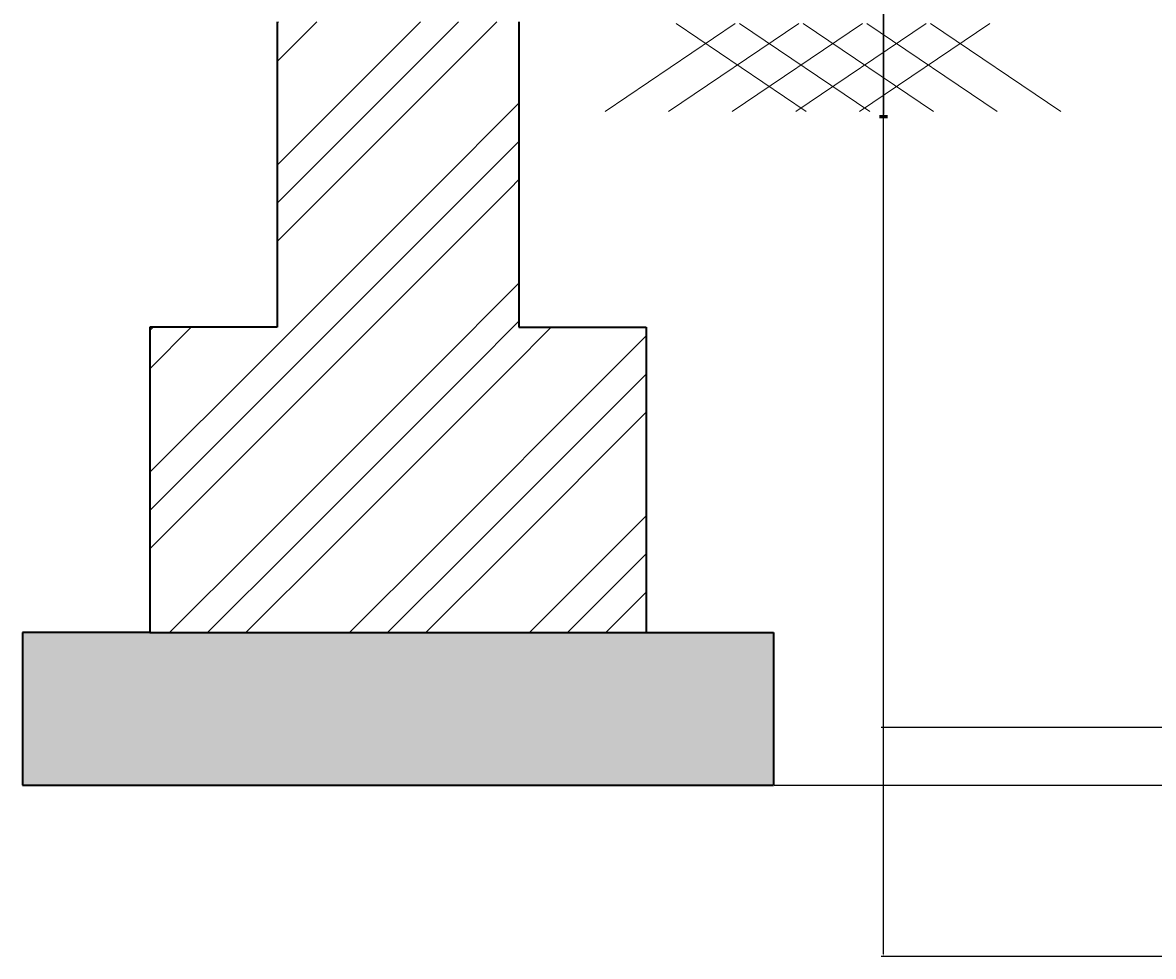
# Model space of a CAD drawing. Units: inches. Extents: x -128 to 854, y -395 to 398.
# Tile 16 of 61: x 279 to 368, y -371 to -298. Entities that reach past the tile are written whole.
import ezdxf

# ---------------------------------------------------------------- set-up
doc = ezdxf.new("R2010")
doc.units = ezdxf.units.IN
doc.header["$MEASUREMENT"] = 0
for name, color, linetype, lineweight in [('A-ANNO-DIMS', 2, 'Continuous', 18), ('A-SECT-PATT', 8, 'Continuous', 13), ('C-GRAD-PATT', 8, 'Continuous', 13), ('S-FNDN', 2, 'Continuous', 35), ('S-FNDN-PATT', 8, 'Continuous', 13)]:
    doc.layers.add(name, color=color, linetype=linetype, lineweight=lineweight)
doc.styles.get("Standard").update_dxf_attribs({"font": 'arial.ttf'})
doc.dimstyles.get("Standard").update_dxf_attribs({"dimtxt": 0.18, "dimasz": 0.18, "dimexe": 0.18, "dimexo": 0.0625, "dimgap": 0.09, "dimtad": 0, "dimtih": 1, "dimtoh": 1, "dimdec": 1, "dimzin": 0, "dimdsep": 46, "dimlunit": 4, "dimtxsty": 'Standard', "dimcen": 0.09, "dimclrd": 1, "dimclre": 2, "dimclrt": 6, "dimadec": 0, "dimazin": 0, "dimtfac": 1, "dimtdec": 1, "dimtofl": 0, "dimtmove": 0, "dimatfit": 3, "dimfxl": 1, "dimtfill": 2, "dimtfillclr": 3, "dimtolj": 1, "dimtzin": 0, "dimarcsym": 0})

# ---------------------------------------------------------------- blocks, each defined once
blk = doc.blocks.new('*D120')
at = {"layer": 'A-ANNO-DIMS', "color": 2, "lineweight": -2, "transparency": 16777216}
for p, q in [((317.902, -178.019), (389.719, -178.019)), ((337.902, -358.019), (389.719, -358.019))]:
    blk.add_line(p, q, dxfattribs=at)
at = {"layer": 'A-ANNO-DIMS', "color": 1, "lineweight": -2, "transparency": 16777216}
for p, q in [((389.539, -178.199), (389.539, -267.837)), ((389.539, -357.839), (389.539, -268.201))]:
    blk.add_line(p, q, dxfattribs=at)
at = {"layer": 'A-ANNO-DIMS', "color": 1, "transparency": 16777216}
for points in [[(389.509, -178.199), (389.569, -178.199), (389.539, -178.019)], [(389.509, -357.839), (389.569, -357.839), (389.539, -358.019)]]:
    blk.add_solid(points, dxfattribs=at)
at = {"layer": 'Defpoints', "color": 0, "transparency": 16777216}
for p in [(317.839, -178.019), (337.839, -358.019), (389.539, -358.019)]:
    blk.add_point(p, dxfattribs=at)
at = {"layer": 'A-ANNO-DIMS', "color": 6, "transparency": 16777216, "insert": (389.539, -268.019), "char_height": 0.18, "attachment_point": 5, "bg_fill": 1, "box_fill_scale": 1.25, "bg_fill_color": 3, "bg_fill_transparency": 0}
blk.add_mtext('\\A1;15\'-0"', dxfattribs=at)
blk = doc.blocks.new('*D134')
at = {"layer": 'A-ANNO-DIMS', "color": 2, "lineweight": -2, "transparency": 16777216}
for p, q in [((418.217, -191.476), (346.3, -191.476)), ((418.217, -371.476), (346.3, -371.476))]:
    blk.add_line(p, q, dxfattribs=at)
at = {"layer": 'A-ANNO-DIMS', "color": 1, "lineweight": -2, "transparency": 16777216}
for p, q in [((346.48, -191.656), (346.48, -281.295)), ((346.48, -371.296), (346.48, -281.658))]:
    blk.add_line(p, q, dxfattribs=at)
at = {"layer": 'A-ANNO-DIMS', "color": 1, "transparency": 16777216}
for points in [[(346.45, -191.656), (346.51, -191.656), (346.48, -191.476)], [(346.45, -371.296), (346.51, -371.296), (346.48, -371.476)]]:
    blk.add_solid(points, dxfattribs=at)
at = {"layer": 'Defpoints', "color": 0, "transparency": 16777216}
for p in [(346.48, -191.476), (418.28, -191.476), (418.28, -371.476)]:
    blk.add_point(p, dxfattribs=at)
at = {"layer": 'A-ANNO-DIMS', "color": 6, "transparency": 16777216, "insert": (346.48, -281.476), "char_height": 0.18, "attachment_point": 5, "bg_fill": 1, "box_fill_scale": 1.25, "bg_fill_color": 3, "bg_fill_transparency": 0}
blk.add_mtext('\\A1;15\'-0"', dxfattribs=at)
blk = doc.blocks.new('*D140')
at = {"layer": 'A-ANNO-DIMS', "color": 2, "lineweight": -2, "transparency": 16777216}
for p, q in [((551.245, -257.476), (346.3, -257.476)), ((551.245, -353.476), (346.3, -353.476))]:
    blk.add_line(p, q, dxfattribs=at)
at = {"layer": 'A-ANNO-DIMS', "color": 1, "lineweight": -2, "transparency": 16777216}
for p, q in [((346.48, -257.656), (346.48, -305.295)), ((346.48, -353.296), (346.48, -305.658))]:
    blk.add_line(p, q, dxfattribs=at)
at = {"layer": 'A-ANNO-DIMS', "color": 1, "transparency": 16777216}
for points in [[(346.45, -257.656), (346.51, -257.656), (346.48, -257.476)], [(346.45, -353.296), (346.51, -353.296), (346.48, -353.476)]]:
    blk.add_solid(points, dxfattribs=at)
at = {"layer": 'Defpoints', "color": 0, "transparency": 16777216}
for p in [(346.48, -257.476), (551.307, -257.476), (551.307, -353.476)]:
    blk.add_point(p, dxfattribs=at)
at = {"layer": 'A-ANNO-DIMS', "color": 6, "transparency": 16777216, "insert": (346.48, -305.476), "char_height": 0.18, "attachment_point": 5, "bg_fill": 1, "box_fill_scale": 1.25, "bg_fill_color": 3, "bg_fill_transparency": 0}
blk.add_mtext('\\A1;8\'-0"', dxfattribs=at)

msp = doc.modelspace()

# ---------------------------------------------------------------- hatches: boundary and pattern name
at = {"layer": 'A-SECT-PATT'}
h = msp.add_hatch(dxfattribs=at)
h.set_pattern_fill('GOST_GROUND', color=256)
h.set_pattern_definition([(45, (0, 0), (14.14214, -9e-16), [20]), (45, (3, 0), (14.14214, -9e-16), [20]), (45, (6, 0), (14.14214, -9e-16), [20])])
h.paths.add_polyline_path([(-27.161, -322.019), (-37.161, -322.019), (-37.161, -298.019), (-56.161, -298.019), (-56.161, -322.019), (-66.161, -322.019), (-66.161, -346.019), (-27.161, -346.019)])
h.paths.add_polyline_path([(170.839, -322.019), (160.839, -322.019), (160.839, -298.019), (155.839, -298.019), (141.839, -298.019), (141.839, -322.019), (131.839, -322.019), (131.839, -346.019), (170.839, -346.019)])
h.paths.add_polyline_path([(327.839, -322.019), (317.839, -322.019), (317.839, -298.019), (312.839, -298.019), (298.839, -298.019), (298.839, -322.019), (288.839, -322.019), (288.839, -346.019), (327.839, -346.019)])
h.paths.add_polyline_path([(-37.161, -274.019), (-56.161, -274.019), (-56.161, -298.019), (-37.161, -298.019)])
h.paths.add_polyline_path([(-37.161, -207.019), (-56.161, -207.019), (-56.161, -226.019), (-37.161, -226.019)])
h.paths.add_polyline_path([(160.839, -274.019), (141.839, -274.019), (141.839, -298.019), (155.839, -298.019), (160.839, -298.019)])
at = {"layer": 'C-GRAD-PATT'}
h = msp.add_hatch(dxfattribs=at)
h.set_pattern_fill('ANSI31', color=256, scale=22.43157, angle=349.1104, style=0)
h.paths.add_polyline_path([(330.046, -298.137), (355.026, -298.137), (344.8, -305.063), (319.82, -305.063)])
h = msp.add_hatch(dxfattribs=at)
h.set_pattern_fill('ANSI31', color=256, scale=22.43157, angle=100.8896, style=0)
h.paths.add_polyline_path([(330.046, -298.137), (355.026, -298.137), (365.252, -305.063), (340.272, -305.063)])
at = {"layer": 'S-FNDN-PATT'}
h = msp.add_hatch(dxfattribs=at)
h.set_pattern_fill('AR-CONC', color=256)
h.paths.add_polyline_path([(-17.161, -346.019), (-27.161, -346.019), (-66.161, -346.019), (-76.161, -346.019), (-76.161, -358.019), (-17.161, -358.019)])
h.paths.add_polyline_path([(180.839, -346.019), (170.839, -346.019), (131.839, -346.019), (121.839, -346.019), (121.839, -358.019), (180.839, -358.019)])
h.paths.add_polyline_path([(337.839, -346.019), (327.839, -346.019), (288.839, -346.019), (278.839, -346.019), (278.839, -358.019), (337.839, -358.019)])

# ---------------------------------------------------------------- linework, layer by layer
at = {"layer": 'S-FNDN'}
for p, q in [((298.839, -298.019), (298.839, -322.019)), ((317.839, -298.019), (317.839, -322.019)), ((298.839, -322.019), (288.839, -322.019)), ((288.839, -322.019), (288.839, -346.019)), ((317.839, -322.019), (327.839, -322.019)), ((327.839, -322.019), (327.839, -346.019)), ((288.839, -346.019), (278.839, -346.019)), ((278.839, -346.019), (278.839, -358.019)), ((288.839, -346.019), (327.839, -346.019)), ((327.839, -346.019), (337.839, -346.019)), ((337.839, -346.019), (337.839, -358.019)), ((278.839, -358.019), (337.839, -358.019))]:
    msp.add_line(p, q, dxfattribs=at)

# ---------------------------------------------------------------- dimensions: what is measured, and where the dimension line sits
at = {"layer": 'A-ANNO-DIMS'}
for base, p1, p2, picture, middle in [((389.539, -358.019), (317.839, -178.019), (337.839, -358.019), '*D120', (389.539, -268.019)), ((346.48, -191.476), (418.28, -371.476), (418.28, -191.476), '*D134', (346.48, -281.476)), ((346.48, -257.476), (551.307, -353.476), (551.307, -257.476), '*D140', (346.48, -305.476))]:
    dim = msp.add_linear_dim(base=base, p1=p1, p2=p2, angle=90, dimstyle='Standard', override={"dimdec": 1, "dimlfac": 1, "dimrnd": 0, "dimzin": 1, "dimdsep": 46, "dimlunit": 4, "dimfrac": 2}, dxfattribs=at)
    dim.commit()
    dim.dimension.update_dxf_attribs({"geometry": picture, "text_midpoint": middle})

doc.saveas('drawing.dxf')
